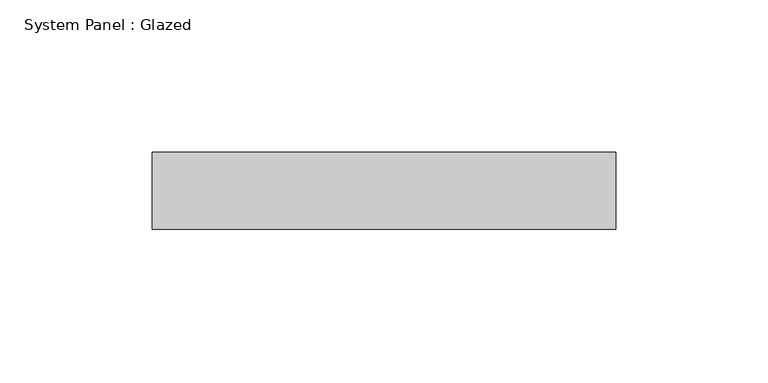
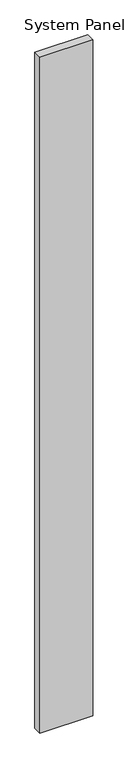
"""IFC4 building model written with IfcOpenShell, lengths in millimetres: plate geometry, System Panel : Glazed."""

from ifc_helpers import new_model, si_unit, origin, origin_with_axes, place, context, project, spatial, polyline, outline, extrude, source, transform, mapped, element, save


def system_panel_glazed_29dc7863(model_context):
    return source(origin(), model_context, "Body", "SweptSolid", [
        extrude(outline(polyline([(76.2, 19.05), (-76.2, 19.05), (-76.2, 44.45), (76.2, 44.45), (76.2, 19.05)])), origin_with_axes(), (0.0, 0.0, 1.0), 2060.8644013),
    ])


if __name__ == "__main__":
    model = new_model("IFC4")
    model_context = context("Model", 3, world=origin())
    ifc_project = project(units=[si_unit("LENGTHUNIT", "METRE", prefix="MILLI")], contexts=[model_context])
    site = spatial("IfcSite", under=ifc_project)
    building = spatial("IfcBuilding", under=site)
    placement = place(None, origin())
    system_panel_glazed_shape = system_panel_glazed_29dc7863(model_context)
    element("IfcPlate", 1, ObjectType="System Panel : Glazed", at=placement, inside=building, context=model_context, shape_type="MappedRepresentation", body=[
        mapped(system_panel_glazed_shape, transform((0.0, 0.0, 0.0), x_axis=(1.0, 0.0, 0.0), y_axis=(0.0, 1.0, 0.0), z_axis=(0.0, 0.0, 1.0))),
    ])
    save(model, "model.ifc")

# Revit data of these elements
# Type "System Panel : Glazed"
#   Construction Type Id = "GSP4R"
#   Analytic Construction = "1/8 in Pilkington single glazing"
#   Visual Light Transmittance = 0.9
#   Solar Heat Gain Coefficient = 0.86
#   Heat Transfer Coefficient (U) = 1.18115 BTU/(h·ft²·°F)
#   Define Thermal Properties by = 1
# Element 1 (IfcPlate, "System Panel : Glazed")
#   Materials on its faces: "Glass"
# Materials
#   "Glass": class "Glass", colour RGB 0 128 192, transparency 0.75, Description = "Soda Lime Glass", Cost = 0
